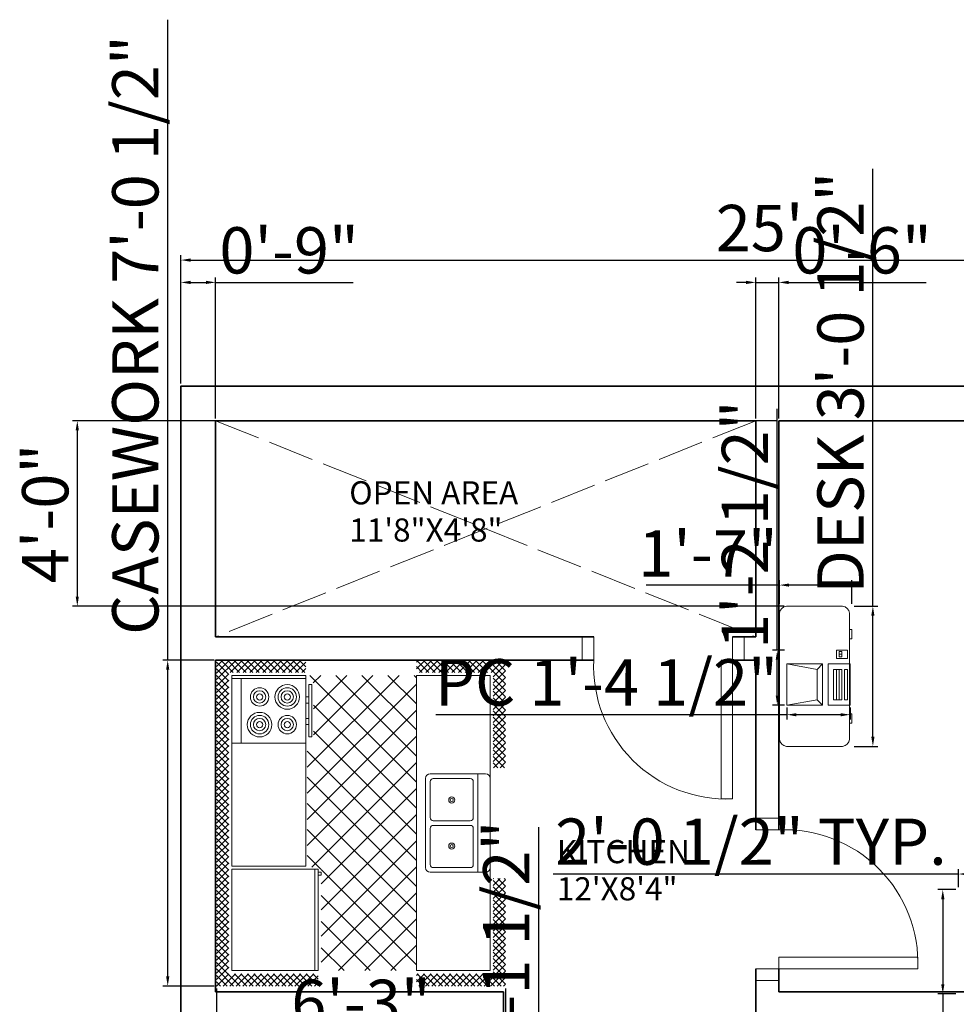
# Model space of a CAD drawing. Units: inches. Extents: x 2446 to 3341, y 462 to 1195.
# Tile 3 of 6: x 2503 to 2746, y 888 to 1143. Entities that reach past the tile are written whole.
import ezdxf

# ---------------------------------------------------------------- set-up
doc = ezdxf.new("R2010")
doc.units = ezdxf.units.IN
doc.linetypes.add('ACAD_ISO02W100', pattern=[15, 12, -3])
for name, color, linetype, lineweight in [('A-ANNO-DIMS', 2, 'Continuous', 18), ('A-AREA-IDEN', 7, 'Continuous', 18), ('A-DOOR', 4, 'Continuous', 18), ('A-EQPM', 9, 'Continuous', 18), ('A-FLOR-FIXT', 9, 'Continuous', 18), ('A-FLOR-OPEN', 8, 'ACAD_ISO02W100', 13), ('A-FURN', 8, 'Continuous', 18), ('A-WALL', 7, 'Continuous', 35), ('C-PROP', 7, 'Continuous', 35)]:
    doc.layers.add(name, color=color, linetype=linetype, lineweight=lineweight)
doc.styles.get("Standard").update_dxf_attribs({"font": 'arial.ttf'})
doc.dimstyles.new('ISO-25', dxfattribs={"dimtxt": 12, "dimasz": 2.5, "dimexe": 1.25, "dimexo": 0.625, "dimtad": 1, "dimdec": 1, "dimlunit": 3, "dimtxsty": 'Standard', "dimcen": 2.5, "dimadec": 0, "dimazin": 0, "dimtfac": 1, "dimtdec": 1, "dimtmove": 0, "dimatfit": 3, "dimfxl": 1, "dimarcsym": 0})

# ---------------------------------------------------------------- blocks, each defined once
blk = doc.blocks.new('Desk - 30 x 60 in.')
for p, q in [((-26.999995, 0), (26.999995, 0)), ((-29.999995, -27), (-29.999995, -3)), ((29.999995, -3), (29.999995, -27)), ((26.999995, -30), (-26.999995, -30)), ((-20.000005, -30), (-20.000005, -31)), ((-20.000005, -31), (-16.000005, -31)), ((-16.000005, -31), (-16.000005, -30)), ((15.999995, -31), (15.999995, -30)), ((19.999995, -31), (15.999995, -31)), ((19.999995, -30), (19.999995, -31))]:
    blk.add_line(p, q)
for centre, start, end in [((-26.499995, -3.5), 98.1301, 171.8699), ((26.499995, -3.5), 8.130102, 81.8699), ((-26.499995, -26.5), 188.1301, 261.8699), ((26.499995, -26.5), 278.1301, 351.8699)]:
    blk.add_arc(centre, 3.535534, start, end)
blk = doc.blocks.new('Computer Terminal')
for p, q in [((-10, 11.5), (5, 11.5)), ((-8, 0.5), (-10, 11.5)), ((-10, -1.5), (-10, 11.5)), ((5, 11.5), (3, 0.5)), ((5, 11.5), (5, -1.5)), ((-10, -1.5), (-8, 0.5)), ((3, 0.5), (-8, 0.5)), ((3, 0.5), (5, -1.5)), ((5, -1.5), (-10, -1.5)), ((-10, -11.5), (-10, -3.5)), ((-10, -3.5), (5, -3.5)), ((5, -3.5), (5, -11.5)), ((-8, -5.5), (-8, -8.5)), ((3, -5.5), (-8, -5.5)), ((3, -6.5), (-8, -6.5)), ((3, -8.5), (3, -5.5)), ((10, -6.5), (7, -6.5)), ((7, -6.5), (7, -10.5)), ((10, -10.5), (10, -6.5)), ((-8, -7.5), (3, -7.5)), ((-8, -8.5), (3, -8.5)), ((-8, -9.5), (-8, -10.5)), ((3, -9.5), (-8, -9.5)), ((-8, -10.5), (3, -10.5)), ((3, -10.5), (3, -9.5)), ((7, -10.5), (10, -10.5)), ((9.5, -7.5), (7.5, -7.5)), ((7.5, -7.5), (7.5, -8.5)), ((7.5, -8.5), (9.5, -8.5)), ((8.5, -7.5), (8.5, -8.5)), ((9.5, -8.5), (9.5, -7.5)), ((5, -11.5), (-10, -11.5))]:
    blk.add_line(p, q)
blk = doc.blocks.new('Kitchen Layout - 7 x 8 ft')
for p, q in [((-5, 81.32), (2.68, 89)), ((-5, 83.44), (0.56, 89)), ((-5, 85.56), (-1.56, 89)), ((-5, 87.68), (-3.68, 89)), ((-1, 84.97), (-5, 88.97)), ((-1, 82.85), (-5, 86.85)), ((1.09, 85), (-2.91, 89)), ((3.21, 85), (-0.79, 89)), ((0.81, 85), (4.81, 89)), ((5.34, 85), (1.34, 89)), ((2.93, 85), (6.93, 89)), ((7.46, 85), (3.46, 89)), ((5.05, 85), (9.05, 89)), ((9.58, 85), (5.58, 89)), ((7.17, 85), (11.17, 89)), ((11.7, 85), (7.7, 89)), ((9.29, 85), (13.29, 89)), ((13.82, 85), (9.82, 89)), ((11.41, 85), (15.41, 89)), ((15.94, 85), (11.94, 89)), ((13.53, 85), (17.53, 89)), ((18.06, 85), (14.06, 89)), ((15.65, 85), (19.65, 89)), ((20.18, 85), (16.18, 89)), ((17.78, 85), (21.78, 89)), ((22.31, 85), (18.31, 89)), ((19.9, 85), (23.9, 89)), ((24.43, 85), (20.43, 89)), ((22.02, 85), (26.02, 89)), ((26.55, 85), (22.55, 89)), ((24.14, 85), (28.14, 89)), ((28.67, 85), (24.67, 89)), ((26.26, 85), (30.26, 89)), ((30.79, 85), (26.79, 89)), ((28.38, 85), (32.38, 89)), ((32.91, 85), (28.91, 89)), ((30.5, 85), (34.5, 89)), ((35.03, 85), (31.03, 89)), ((32.63, 85), (36.63, 89)), ((37.16, 85), (33.16, 89)), ((34.75, 85), (38.75, 89)), ((39.28, 85), (35.28, 89)), ((36.87, 85), (40.87, 89)), ((41.4, 85), (37.4, 89)), ((38.99, 85), (42.99, 89)), ((43.52, 85), (39.52, 89)), ((41.11, 85), (45.11, 89)), ((45.64, 85), (41.64, 89)), ((43.23, 85), (47.23, 89)), ((47.76, 85), (43.76, 89)), ((45.35, 85), (49.35, 89)), ((49.88, 85), (45.88, 89)), ((47.47, 85), (51.47, 89)), ((52, 85), (48, 89)), ((49.6, 85), (53.6, 89)), ((54.13, 85), (50.13, 89)), ((51.72, 85), (55.72, 89)), ((56.25, 85), (52.25, 89)), ((53.84, 85), (57.84, 89)), ((58.37, 85), (54.37, 89)), ((55.96, 85), (59.96, 89)), ((60.49, 85), (56.49, 89)), ((58.08, 85), (62.08, 89)), ((62.61, 85), (58.61, 89)), ((60.2, 85), (64.2, 89)), ((64.73, 85), (60.73, 89)), ((62.32, 85), (66.32, 89)), ((66.85, 85), (62.85, 89)), ((64.45, 85), (68.45, 89)), ((68.97, 85), (64.97, 89)), ((66.57, 85), (70.57, 89)), ((71.1, 85), (67.1, 89)), ((68.69, 85), (72.69, 89)), ((73.22, 85), (69.22, 89)), ((70.81, 85), (74.81, 89)), ((75.34, 85), (71.34, 89)), ((72.93, 85), (76.93, 89)), ((77.46, 85), (73.46, 89)), ((75.05, 85), (79.05, 89)), ((79.58, 85), (75.58, 89)), ((77.17, 85), (81.17, 89)), ((81.7, 85), (77.7, 89)), ((79.29, 85), (83.29, 89)), ((83.82, 85), (79.82, 89)), ((81.42, 85), (85.42, 89)), ((85.95, 85), (81.95, 89)), ((83.54, 85), (87.54, 89)), ((88.07, 85), (84.07, 89)), ((85.66, 85), (89.66, 89)), ((90.19, 85), (86.19, 89)), ((87.78, 85), (91.78, 89)), ((92.31, 85), (88.31, 89)), ((89.9, 85), (93.9, 89)), ((94.43, 85), (90.43, 89)), ((92.02, 85), (96.02, 89)), ((96.55, 85), (92.55, 89)), ((94.14, 85), (98.14, 89)), ((101, 82.67), (94.67, 89)), ((96.27, 85), (100.27, 89)), ((101, 84.79), (96.79, 89)), ((97, 83.61), (101, 87.61)), ((101, 86.92), (98.92, 89)), ((-1, 80.73), (-5, 84.73)), ((34, 84), (96, 84)), ((34, 60), (34, 84)), ((96, 84), (96, 60)), ((97, 81.49), (101, 85.49)), ((101, 80.55), (97, 84.55)), ((97, 79.37), (101, 83.37)), ((-5, 79.19), (-1, 83.19)), ((-1, 78.61), (-5, 82.61)), ((-5, 77.07), (-1, 81.07)), ((-1, 76.49), (-5, 80.49)), ((74, 81), (95, 81)), ((101, 78.43), (97, 82.43)), ((97, 77.25), (101, 81.25)), ((101, 76.31), (97, 80.31)), ((-5, 74.95), (-1, 78.95)), ((-1, 74.36), (-5, 78.36)), ((97, 75.13), (101, 79.13)), ((101, 74.19), (97, 78.19)), ((97, 73.01), (101, 77.01)), ((-5, 72.83), (-1, 76.83)), ((-1, 72.24), (-5, 76.24)), ((-5, 70.71), (-1, 74.71)), ((-1, 70.12), (-5, 74.12)), ((101, 72.07), (97, 76.07)), ((97, 70.89), (101, 74.89)), ((101, 69.95), (97, 73.95)), ((-5, 68.59), (-1, 72.59)), ((-1, 68), (-5, 72)), ((-5, 66.47), (-1, 70.47)), ((97, 68.76), (101, 72.76)), ((101, 67.82), (97, 71.82)), ((97, 66.64), (101, 70.64)), ((-1, 65.88), (-5, 69.88)), ((-5, 64.35), (-1, 68.35)), ((-1, 63.76), (-5, 67.76)), ((101, 65.7), (97, 69.7)), ((97, 64.52), (101, 68.52)), ((101, 63.58), (97, 67.58)), ((-5, 62.22), (-1, 66.22)), ((-1, 61.64), (-5, 65.64)), ((-5, 60.1), (-1, 64.1)), ((97, 62.4), (101, 66.4)), ((101, 61.46), (97, 65.46)), ((97, 60.28), (101, 64.28)), ((-1, 59.52), (-5, 63.52)), ((-5, 57.98), (-1, 61.98)), ((-1, 57.39), (-5, 61.39)), ((100.34, 60), (97, 63.34)), ((98.22, 60), (97, 61.22)), ((98.84, 60), (101, 62.16)), ((-1.73, 56), (-5, 59.27)), ((-4.86, 56), (-1, 59.86)), ((-2.74, 56), (-1, 57.74)), ((10.4, 24), (45.9, 59.5)), ((18.88, 24), (54.38, 59.5)), ((27.37, 24), (62.87, 59.5)), ((33.03, 55.11), (37.41, 59.5)), ((67.71, 24), (33.68, 58.04)), ((96, 60), (34, 60)), ((35.85, 24), (71.35, 59.5)), ((76.2, 24), (40.7, 59.5)), ((84.68, 24), (49.18, 59.5)), ((93.17, 24), (57.67, 59.5)), ((61.31, 24), (96, 58.69)), ((96, 29.65), (66.15, 59.5)), ((80, 60), (80, 59)), ((82, 59), (82, 60)), ((87, 59), (87, 60)), ((89, 60), (89, 59)), ((100.96, 60), (101, 60.04)), ((-3.85, 56), (-5, 57.15)), ((0, 57), (33, 57)), ((0, 30.57), (24.43, 55)), ((0, 39.06), (15.94, 55)), ((0, 47.54), (7.46, 55)), ((1.91, 24), (32.91, 55)), ((33.77, 24), (2.77, 55)), ((42.26, 24), (11.26, 55)), ((50.74, 24), (19.74, 55)), ((59.23, 24), (28.23, 55)), ((31, 55), (31, 56)), ((32, 55), (31, 55)), ((32, 56), (32, 55)), ((44.34, 24), (77.84, 57.5)), ((52.82, 24), (86.32, 57.5)), ((96, 38.14), (76.64, 57.5)), ((96, 46.63), (85.13, 57.5)), ((96, 55.11), (93.57, 57.54)), ((25.29, 24), (0, 49.29)), ((69.79, 24), (96, 50.21)), ((78.28, 24), (96, 41.72)), ((16.8, 24), (0, 40.8)), ((8.32, 24), (0, 32.32)), ((86.76, 24), (96, 33.24)), ((-5, 21.92), (-2.92, 24)), ((-5, 19.8), (-1, 23.8)), ((-1, 19.21), (-5, 23.21)), ((-1, 21.33), (-3.67, 24)), ((-1, 23.45), (-1.55, 24)), ((0, 24), (96, 24)), ((0, 0), (0, 24)), ((95.25, 24), (96, 24.75)), ((96, 24), (96, 0)), ((97, 22.1), (98.9, 24)), ((97, 19.97), (101, 23.97)), ((101, 19.03), (97, 23.03)), ((101, 21.16), (98.16, 24)), ((101, 23.28), (100.28, 24)), ((-5, 17.68), (-1, 21.68)), ((-1, 17.09), (-5, 21.09)), ((-5, 15.55), (-1, 19.55)), ((97, 17.85), (101, 21.85)), ((101, 16.91), (97, 20.91)), ((97, 15.73), (101, 19.73)), ((-1, 14.97), (-5, 18.97)), ((-5, 13.43), (-1, 17.43)), ((-1, 12.85), (-5, 16.85)), ((47.25, 6.5), (47.25, 18.5)), ((48.75, 18.5), (48.75, 6.5)), ((101, 14.79), (97, 18.79)), ((97, 13.61), (101, 17.61)), ((101, 12.67), (97, 16.67)), ((-5, 11.31), (-1, 15.31)), ((-1, 10.73), (-5, 14.73)), ((-5, 9.19), (-1, 13.19)), ((97, 11.49), (101, 15.49)), ((101, 10.55), (97, 14.55)), ((97, 9.37), (101, 13.37)), ((-1, 8.6), (-5, 12.6)), ((-5, 7.07), (-1, 11.07)), ((-1, 6.48), (-5, 10.48)), ((101, 8.43), (97, 12.43)), ((97, 7.25), (101, 11.25)), ((101, 6.31), (97, 10.31)), ((-5, 4.95), (-1, 8.95)), ((-1, 4.36), (-5, 8.36)), ((-5, 2.83), (-1, 6.83)), ((97, 5.12), (101, 9.12)), ((101, 4.18), (97, 8.18)), ((97, 3), (101, 7)), ((-1, 2.24), (-5, 6.24)), ((-5, 0.71), (-1, 4.71)), ((-1, 0.12), (-5, 4.12)), ((64, 4), (32, 4)), ((101, 2.06), (97, 6.06)), ((97, 0.88), (101, 4.88)), ((101, -0.06), (97, 3.94)), ((-5, -1.42), (-1, 2.58)), ((2, -5), (-5, 2)), ((-5, -3.54), (-1, 0.46)), ((96, 0), (0, 0)), ((93.24, -5), (101, 2.76)), ((95.36, -5), (101, 0.64)), ((101, -2.18), (97, 1.82)), ((-0.12, -5), (-5, -0.12)), ((-2.25, -5), (-5, -2.25)), ((-4.34, -5), (-0.34, -1)), ((-2.22, -5), (1.78, -1)), ((-0.1, -5), (3.9, -1)), ((4.12, -5), (0.12, -1)), ((2.02, -5), (6.02, -1)), ((6.24, -5), (2.24, -1)), ((4.14, -5), (8.14, -1)), ((8.36, -5), (4.36, -1)), ((6.27, -5), (10.27, -1)), ((10.48, -5), (6.48, -1)), ((8.39, -5), (12.39, -1)), ((12.6, -5), (8.6, -1)), ((10.51, -5), (14.51, -1)), ((14.73, -5), (10.73, -1)), ((12.63, -5), (16.63, -1)), ((16.85, -5), (12.85, -1)), ((14.75, -5), (18.75, -1)), ((18.97, -5), (14.97, -1)), ((16.87, -5), (20.87, -1)), ((21.09, -5), (17.09, -1)), ((18.99, -5), (22.99, -1)), ((23.21, -5), (19.21, -1)), ((21.11, -5), (25.11, -1)), ((25.33, -5), (21.33, -1)), ((23.24, -5), (27.24, -1)), ((27.45, -5), (23.45, -1)), ((25.36, -5), (29.36, -1)), ((29.57, -5), (25.57, -1)), ((27.48, -5), (30, -2.48)), ((30, -3.3), (27.7, -1)), ((30, -1.18), (29.82, -1)), ((66, -2.54), (67.54, -1)), ((66, -4.66), (69.66, -1)), ((69.88, -5), (66, -1.12)), ((67.78, -5), (71.78, -1)), ((72, -5), (68, -1)), ((69.9, -5), (73.9, -1)), ((74.12, -5), (70.12, -1)), ((72.03, -5), (76.03, -1)), ((76.24, -5), (72.24, -1)), ((74.15, -5), (78.15, -1)), ((78.36, -5), (74.36, -1)), ((76.27, -5), (80.27, -1)), ((80.49, -5), (76.49, -1)), ((78.39, -5), (82.39, -1)), ((82.61, -5), (78.61, -1)), ((80.51, -5), (84.51, -1)), ((84.73, -5), (80.73, -1)), ((82.63, -5), (86.63, -1)), ((86.85, -5), (82.85, -1)), ((84.75, -5), (88.75, -1)), ((88.97, -5), (84.97, -1)), ((86.88, -5), (90.88, -1)), ((91.09, -5), (87.09, -1)), ((89, -5), (93, -1)), ((93.21, -5), (89.21, -1)), ((91.12, -5), (95.12, -1)), ((95.34, -5), (91.34, -1)), ((97.46, -5), (93.46, -1)), ((99.58, -5), (95.58, -1)), ((101, -4.3), (97, -0.3)), ((97.48, -5), (101, -1.48)), ((-4.37, -5), (-5, -4.37)), ((29.6, -5), (30, -4.6)), ((67.76, -5), (66, -3.24)), ((99.6, -5), (101, -3.6))]:
    blk.add_line(p, q)
for points in [[(0, 56), (0, 84), (33, 84), (33, 56)], [(74, 60), (74, 84), (95, 84), (95, 60)], [(76, 58), (76, 59), (93, 59), (93, 58)]]:
    blk.add_lwpolyline(points, close=True)
for points in [[(32, 1.5), (32, 19.5)], [(33.5, 21), (62.5, 21)], [(34.5, 19.5), (46.25, 19.5)], [(49.75, 19.5), (61.5, 19.5)], [(64, 19.5), (64, 1.5)], [(33.5, 6.5), (33.5, 18.5)], [(62.5, 18.5), (62.5, 6.5)], [(46.25, 5.5), (34.5, 5.5)], [(61.5, 5.5), (49.75, 5.5)], [(62.5, 0), (33.5, 0)]]:
    blk.add_lwpolyline(points)
for centre, radius in [((80, 75), 4), ((80, 75), 3), ((80, 75), 2), ((89, 75), 3), ((89, 75), 2), ((80, 75), 1), ((89, 75), 1), ((80, 66), 3), ((80, 66), 2), ((89, 66), 4), ((89, 66), 3), ((89, 66), 2), ((80, 66), 1), ((89, 66), 1), ((40.5, 12.5), 1), ((40.5, 12.5), 0.5), ((55.5, 12.5), 1), ((55.5, 12.5), 0.5)]:
    blk.add_circle(centre, radius)
for centre, radius, start, end in [((33.5, 19.5), 1.5, 90, 180), ((34.5, 18.5), 1, 90, 180), ((46.25, 18.5), 1, 0, 90), ((49.75, 18.5), 1, 90, 180), ((61.5, 18.5), 1, 0, 90), ((62.5, 19.5), 1.5, 0, 90), ((34.5, 6.5), 1, 180, 270), ((46.25, 6.5), 1, 270, 0), ((49.75, 6.5), 1, 180, 270), ((61.5, 6.5), 1, 270, 0), ((33.5, 1.5), 1.5, 180, 270), ((62.5, 1.5), 1.5, 270, 0)]:
    blk.add_arc(centre, radius, start, end)
blk = doc.blocks.new('*D17')
at = {"layer": 'A-ANNO-DIMS', "color": 0, "lineweight": -2, "transparency": 16777216}
for p, q in [((2544.62, 1048.59), (2544.62, 1081.85)), ((2844.62, 1048.59), (2844.62, 1081.85)), ((2547.12, 1080.6), (2842.12, 1080.6))]:
    blk.add_line(p, q, dxfattribs=at)
at = {"layer": 'A-ANNO-DIMS', "color": 0, "transparency": 16777216}
for points in [[(2547.12, 1081.02), (2547.12, 1080.18), (2544.62, 1080.6)], [(2842.12, 1081.02), (2842.12, 1080.18), (2844.62, 1080.6)]]:
    blk.add_solid(points, dxfattribs=at)
at = {"layer": 'Defpoints', "color": 0, "transparency": 16777216}
for p in [(2844.62, 1080.6), (2544.62, 1047.97), (2844.62, 1047.97)]:
    blk.add_point(p, dxfattribs=at)
at = {"layer": 'A-ANNO-DIMS', "color": 0, "transparency": 16777216, "insert": (2694.62, 1087.35), "char_height": 12, "attachment_point": 5}
blk.add_mtext("25'", dxfattribs=at)
blk = doc.blocks.new('DOOR-SWING-36IN')
for p, q in [((6, 42), (0, 42)), ((6, 39), (0, 39)), ((6, 3), (0, 3)), ((6, 0), (0, 0))]:
    blk.add_line(p, q)
blk.add_lwpolyline([(6, 3), (42, 3), (42, 6), (6, 6)], close=True)
blk.add_arc((7.5, 4.5), 34.53, 357.5104, 92.4896)
blk = doc.blocks.new('*D33')
at = {"layer": 'A-ANNO-DIMS', "color": 0, "lineweight": -2, "transparency": 16777216}
for p, q in [((2745.53, 917.47), (2740.86, 917.47)), ((2742.11, 914.97), (2742.11, 892.97)), ((2745.53, 890.47), (2740.86, 890.47)), ((2742.11, 890.47), (2742.11, 737.82))]:
    blk.add_line(p, q, dxfattribs=at)
at = {"layer": 'A-ANNO-DIMS', "color": 0, "transparency": 16777216}
for points in [[(2741.69, 914.97), (2742.53, 914.97), (2742.11, 917.47)], [(2741.69, 892.97), (2742.53, 892.97), (2742.11, 890.47)]]:
    blk.add_solid(points, dxfattribs=at)
at = {"layer": 'Defpoints', "color": 0, "transparency": 16777216}
for p in [(2746.16, 917.47), (2742.11, 890.47), (2746.16, 890.47)]:
    blk.add_point(p, dxfattribs=at)
at = {"layer": 'A-ANNO-DIMS', "color": 0, "transparency": 16777216, "insert": (2735.27, 812.89), "char_height": 12, "attachment_point": 5, "rotation": 90}
blk.add_mtext('ROCKER 2\'-3" TYP.', dxfattribs=at)
blk = doc.blocks.new('*D34')
at = {"layer": 'A-ANNO-DIMS', "color": 0, "lineweight": -2, "transparency": 16777216}
for p, q in [((2746.16, 921.52), (2641.1, 921.52)), ((2746.16, 918.09), (2746.16, 922.77)), ((2768.09, 921.52), (2748.66, 921.52)), ((2770.59, 918.09), (2770.59, 922.77))]:
    blk.add_line(p, q, dxfattribs=at)
at = {"layer": 'A-ANNO-DIMS', "color": 0, "transparency": 16777216}
for points in [[(2748.66, 921.94), (2748.66, 921.1), (2746.16, 921.52)], [(2768.09, 921.94), (2768.09, 921.1), (2770.59, 921.52)]]:
    blk.add_solid(points, dxfattribs=at)
at = {"layer": 'Defpoints', "color": 0, "transparency": 16777216}
for p in [(2746.16, 921.52), (2746.16, 917.47), (2770.59, 917.47)]:
    blk.add_point(p, dxfattribs=at)
at = {"layer": 'A-ANNO-DIMS', "color": 0, "transparency": 16777216, "insert": (2692.38, 928.35), "char_height": 12, "attachment_point": 5}
blk.add_mtext('2\'-0 1/2" TYP.', dxfattribs=at)
blk = doc.blocks.new('*D41')
at = {"layer": 'A-ANNO-DIMS', "color": 0, "lineweight": -2, "transparency": 16777216}
for p, q in [((2723.99, 990.93), (2723.99, 1104.25)), ((2719.16, 990.93), (2725.24, 990.93)), ((2723.99, 957.09), (2723.99, 988.43)), ((2719.16, 954.59), (2725.24, 954.59))]:
    blk.add_line(p, q, dxfattribs=at)
at = {"layer": 'A-ANNO-DIMS', "color": 0, "transparency": 16777216}
for points in [[(2723.57, 988.43), (2724.4, 988.43), (2723.99, 990.93)], [(2723.57, 957.09), (2724.4, 957.09), (2723.99, 954.59)]]:
    blk.add_solid(points, dxfattribs=at)
at = {"layer": 'Defpoints', "color": 0, "transparency": 16777216}
for p in [(2718.54, 990.93), (2723.99, 990.93), (2718.54, 954.59)]:
    blk.add_point(p, dxfattribs=at)
at = {"layer": 'A-ANNO-DIMS', "color": 0, "transparency": 16777216, "insert": (2717.15, 1048.84), "char_height": 12, "attachment_point": 5, "rotation": 90}
blk.add_mtext('DESK 3\'-0 1/2"', dxfattribs=at)
blk = doc.blocks.new('*D42')
at = {"layer": 'A-ANNO-DIMS', "color": 0, "lineweight": -2, "transparency": 16777216}
for p, q in [((2699.76, 991.56), (2699.76, 997.64)), ((2718.54, 991.56), (2718.54, 997.64)), ((2699.76, 996.39), (2665.24, 996.39)), ((2716.04, 996.39), (2702.26, 996.39))]:
    blk.add_line(p, q, dxfattribs=at)
at = {"layer": 'A-ANNO-DIMS', "color": 0, "transparency": 16777216}
for points in [[(2702.26, 996.8), (2702.26, 995.97), (2699.76, 996.39)], [(2716.04, 996.8), (2716.04, 995.97), (2718.54, 996.39)]]:
    blk.add_solid(points, dxfattribs=at)
at = {"layer": 'Defpoints', "color": 0, "transparency": 16777216}
for p in [(2699.76, 996.39), (2699.76, 990.93), (2718.54, 990.93)]:
    blk.add_point(p, dxfattribs=at)
at = {"layer": 'A-ANNO-DIMS', "color": 0, "transparency": 16777216, "insert": (2681.25, 1003.03), "char_height": 12, "attachment_point": 5}
blk.add_mtext('1\'-7"', dxfattribs=at)
blk = doc.blocks.new('*D45')
at = {"layer": 'A-ANNO-DIMS', "color": 0, "lineweight": -2, "transparency": 16777216}
for p, q in [((2701.68, 964.63), (2701.68, 961.55)), ((2718.1, 964.63), (2718.1, 961.55)), ((2701.68, 962.8), (2610.72, 962.8)), ((2715.6, 962.8), (2704.18, 962.8))]:
    blk.add_line(p, q, dxfattribs=at)
at = {"layer": 'A-ANNO-DIMS', "color": 0, "transparency": 16777216}
for points in [[(2704.18, 963.21), (2704.18, 962.38), (2701.68, 962.8)], [(2715.6, 963.21), (2715.6, 962.38), (2718.1, 962.8)]]:
    blk.add_solid(points, dxfattribs=at)
at = {"layer": 'Defpoints', "color": 0, "transparency": 16777216}
for p in [(2701.68, 965.26), (2718.1, 965.26), (2701.68, 962.8)]:
    blk.add_point(p, dxfattribs=at)
at = {"layer": 'A-ANNO-DIMS', "color": 0, "transparency": 16777216, "insert": (2654.95, 969.63), "char_height": 12, "attachment_point": 5}
blk.add_mtext('PC 1\'-4 1/2"', dxfattribs=at)
blk = doc.blocks.new('*D46')
at = {"layer": 'A-ANNO-DIMS', "color": 0, "lineweight": -2, "transparency": 16777216}
for p, q in [((2699.21, 979.54), (2699.21, 1042.02)), ((2701.05, 979.54), (2697.96, 979.54)), ((2699.21, 967.76), (2699.21, 977.04)), ((2701.05, 965.26), (2697.96, 965.26))]:
    blk.add_line(p, q, dxfattribs=at)
at = {"layer": 'A-ANNO-DIMS', "color": 0, "transparency": 16777216}
for points in [[(2698.8, 977.04), (2699.63, 977.04), (2699.21, 979.54)], [(2698.8, 967.76), (2699.63, 967.76), (2699.21, 965.26)]]:
    blk.add_solid(points, dxfattribs=at)
at = {"layer": 'Defpoints', "color": 0, "transparency": 16777216}
for p in [(2699.21, 979.54), (2701.68, 979.54), (2701.68, 965.26)]:
    blk.add_point(p, dxfattribs=at)
at = {"layer": 'A-ANNO-DIMS', "color": 0, "transparency": 16777216, "insert": (2692.38, 1012.03), "char_height": 12, "attachment_point": 5, "rotation": 90}
blk.add_mtext('1\'-2 1/2"', dxfattribs=at)
blk = doc.blocks.new('*D54')
at = {"layer": 'A-ANNO-DIMS', "color": 0, "lineweight": -2, "transparency": 16777216}
for p, q in [((2637.36, 870.08), (2637.36, 933.69)), ((2628.68, 870.08), (2638.61, 870.08)), ((2637.36, 835.1), (2637.36, 867.58)), ((2628.68, 832.6), (2638.61, 832.6))]:
    blk.add_line(p, q, dxfattribs=at)
at = {"layer": 'A-ANNO-DIMS', "color": 0, "transparency": 16777216}
for points in [[(2636.94, 867.58), (2637.77, 867.58), (2637.36, 870.08)], [(2636.94, 835.1), (2637.77, 835.1), (2637.36, 832.6)]]:
    blk.add_solid(points, dxfattribs=at)
at = {"layer": 'Defpoints', "color": 0, "transparency": 16777216}
for p in [(2628.06, 870.08), (2637.36, 870.08), (2628.06, 832.6)]:
    blk.add_point(p, dxfattribs=at)
at = {"layer": 'A-ANNO-DIMS', "color": 0, "transparency": 16777216, "insert": (2630.52, 903.14), "char_height": 12, "attachment_point": 5, "rotation": 90}
blk.add_mtext('3\'-1 1/2"', dxfattribs=at)
blk = doc.blocks.new('*D55')
at = {"layer": 'A-ANNO-DIMS', "color": 0, "lineweight": -2, "transparency": 16777216}
for p, q in [((2541.2, 976.96), (2541.2, 1142.89)), ((2553.25, 976.96), (2539.95, 976.96)), ((2541.2, 895), (2541.2, 974.46)), ((2553.25, 892.5), (2539.95, 892.5))]:
    blk.add_line(p, q, dxfattribs=at)
at = {"layer": 'A-ANNO-DIMS', "color": 0, "transparency": 16777216}
for points in [[(2540.79, 974.46), (2541.62, 974.46), (2541.2, 976.96)], [(2540.79, 895), (2541.62, 895), (2541.2, 892.5)]]:
    blk.add_solid(points, dxfattribs=at)
at = {"layer": 'Defpoints', "color": 0, "transparency": 16777216}
for p in [(2541.2, 976.96), (2553.87, 976.96), (2553.87, 892.5)]:
    blk.add_point(p, dxfattribs=at)
at = {"layer": 'A-ANNO-DIMS', "color": 0, "transparency": 16777216, "insert": (2534.37, 1061.18), "char_height": 12, "attachment_point": 5, "rotation": 90}
blk.add_mtext('CASEWORK 7\'-0 1/2"', dxfattribs=at)
blk = doc.blocks.new('*D56')
at = {"layer": 'A-ANNO-DIMS', "color": 0, "lineweight": -2, "transparency": 16777216}
for p, q in [((2553.87, 891.87), (2553.87, 878.58)), ((2628.78, 891.87), (2628.78, 878.58)), ((2626.28, 879.83), (2556.37, 879.83))]:
    blk.add_line(p, q, dxfattribs=at)
at = {"layer": 'A-ANNO-DIMS', "color": 0, "transparency": 16777216}
for points in [[(2556.37, 880.24), (2556.37, 879.41), (2553.87, 879.83)], [(2626.28, 880.24), (2626.28, 879.41), (2628.78, 879.83)]]:
    blk.add_solid(points, dxfattribs=at)
at = {"layer": 'Defpoints', "color": 0, "transparency": 16777216}
for p in [(2553.87, 892.5), (2628.78, 892.5), (2553.87, 879.83)]:
    blk.add_point(p, dxfattribs=at)
at = {"layer": 'A-ANNO-DIMS', "color": 0, "transparency": 16777216, "insert": (2591.32, 886.58), "char_height": 12, "attachment_point": 5}
blk.add_mtext('6\'-3"', dxfattribs=at)
blk = doc.blocks.new('*D67')
at = {"layer": 'A-ANNO-DIMS', "color": 0, "lineweight": -2, "transparency": 16777216}
for p, q in [((2544.62, 1048.59), (2544.62, 1076.07)), ((2547.12, 1074.82), (2551.12, 1074.82)), ((2553.62, 1039.59), (2553.62, 1076.07)), ((2553.62, 1074.82), (2589.27, 1074.82))]:
    blk.add_line(p, q, dxfattribs=at)
at = {"layer": 'A-ANNO-DIMS', "color": 0, "transparency": 16777216}
for points in [[(2547.12, 1075.24), (2547.12, 1074.4), (2544.62, 1074.82)], [(2551.12, 1075.24), (2551.12, 1074.4), (2553.62, 1074.82)]]:
    blk.add_solid(points, dxfattribs=at)
at = {"layer": 'Defpoints', "color": 0, "transparency": 16777216}
for p in [(2553.62, 1074.82), (2544.62, 1047.97), (2553.62, 1038.97)]:
    blk.add_point(p, dxfattribs=at)
at = {"layer": 'A-ANNO-DIMS', "color": 0, "transparency": 16777216, "insert": (2572.69, 1081.57), "char_height": 12, "attachment_point": 5}
blk.add_mtext('0\'-9"', dxfattribs=at)
blk = doc.blocks.new('*D68')
at = {"layer": 'A-ANNO-DIMS', "color": 0, "lineweight": -2, "transparency": 16777216}
for p, q in [((2691.12, 1074.82), (2688.62, 1074.82)), ((2693.62, 1039.59), (2693.62, 1076.07)), ((2693.62, 1074.82), (2699.62, 1074.82)), ((2699.62, 1039.59), (2699.62, 1076.07)), ((2702.12, 1074.82), (2737.77, 1074.82))]:
    blk.add_line(p, q, dxfattribs=at)
at = {"layer": 'A-ANNO-DIMS', "color": 0, "transparency": 16777216}
for points in [[(2691.12, 1075.24), (2691.12, 1074.4), (2693.62, 1074.82)], [(2702.12, 1075.24), (2702.12, 1074.4), (2699.62, 1074.82)]]:
    blk.add_solid(points, dxfattribs=at)
at = {"layer": 'Defpoints', "color": 0, "transparency": 16777216}
for p in [(2699.62, 1074.82), (2693.62, 1038.97), (2699.62, 1038.97)]:
    blk.add_point(p, dxfattribs=at)
at = {"layer": 'A-ANNO-DIMS', "color": 0, "transparency": 16777216, "insert": (2721.19, 1081.57), "char_height": 12, "attachment_point": 5}
blk.add_mtext('0\'-6"', dxfattribs=at)
blk = doc.blocks.new('*D77')
at = {"layer": 'A-ANNO-DIMS', "color": 0, "lineweight": -2, "transparency": 16777216}
for p, q in [((2698.99, 1038.97), (2516.52, 1038.97)), ((2517.77, 1036.47), (2517.77, 993.43)), ((2700.95, 990.93), (2516.52, 990.93))]:
    blk.add_line(p, q, dxfattribs=at)
at = {"layer": 'A-ANNO-DIMS', "color": 0, "transparency": 16777216}
for points in [[(2517.35, 1036.47), (2518.18, 1036.47), (2517.77, 1038.97)], [(2517.35, 993.43), (2518.18, 993.43), (2517.77, 990.93)]]:
    blk.add_solid(points, dxfattribs=at)
at = {"layer": 'Defpoints', "color": 0, "transparency": 16777216}
for p in [(2699.62, 1038.97), (2517.77, 990.93), (2701.57, 990.93)]:
    blk.add_point(p, dxfattribs=at)
at = {"layer": 'A-ANNO-DIMS', "color": 0, "transparency": 16777216, "insert": (2511.01, 1014.95), "char_height": 12, "attachment_point": 5, "rotation": 90}
blk.add_mtext('4\'-0"', dxfattribs=at)

msp = doc.modelspace()

# ---------------------------------------------------------------- linework, layer by layer
at = {"layer": 'A-FLOR-OPEN'}
for p, q in [((2553.62, 1038.97), (2693.62, 982.97)), ((2693.62, 1038.97), (2553.62, 982.97))]:
    msp.add_line(p, q, dxfattribs=at)
at = {"layer": 'A-WALL'}
for p, q in [((2553.62, 1038.97), (2553.62, 982.97)), ((2693.62, 1038.97), (2553.62, 1038.97)), ((2693.62, 1038.97), (2693.62, 982.97)), ((2835.62, 1038.97), (2699.62, 1038.97)), ((2699.62, 1038.97), (2699.62, 932.97)), ((2651.62, 982.97), (2553.62, 982.97)), ((2693.62, 982.97), (2687.62, 982.97)), ((2553.62, 976.97), (2553.62, 890.97)), ((2651.62, 976.97), (2553.62, 976.97)), ((2693.62, 976.97), (2687.62, 976.97)), ((2693.62, 976.97), (2693.62, 932.97)), ((2693.62, 896.97), (2693.62, 890.97)), ((2699.62, 896.97), (2699.62, 890.97)), ((2628.27, 890.97), (2553.62, 890.97)), ((2628.27, 890.97), (2628.27, 884.97)), ((2693.62, 890.97), (2693.62, 884.97)), ((2835.62, 890.97), (2699.62, 890.97))]:
    msp.add_line(p, q, dxfattribs=at)
at = {"layer": 'C-PROP'}
msp.add_lwpolyline([(2544.62, 567.97), (2844.62, 567.97), (2844.62, 1047.97), (2544.62, 1047.97)], close=True, dxfattribs=at)

# ---------------------------------------------------------------- block references
at = {"layer": 'A-DOOR', "extrusion": (0, 0, -1), "zscale": -1, "rotation": 269.999999999998}
msp.add_blockref('DOOR-SWING-36IN', (-2690.62, 982.97), dxfattribs=at)
at = {"layer": 'A-DOOR'}
msp.add_blockref('DOOR-SWING-36IN', (2693.62, 893.97), dxfattribs=at)
at = {"layer": 'A-EQPM', "xscale": 0.7141072854781568, "yscale": 0.7141072854781568, "zscale": 0.7141072854781568, "rotation": 90}
msp.add_blockref('Computer Terminal', (2709.89, 972.4), dxfattribs=at)
at = {"layer": 'A-FLOR-FIXT', "xscale": 0.7968505236229118, "yscale": 0.7968505236229118, "zscale": 0.7968505236229118, "rotation": 90}
msp.add_blockref('Kitchen Layout - 7 x 8 ft', (2624.79, 896.48), dxfattribs=at)
at = {"layer": 'A-FURN', "xscale": 0.6057898034963493, "yscale": 0.6057898034963493, "zscale": 0.6057898034963493, "rotation": 90}
msp.add_blockref('Desk - 30 x 60 in.', (2699.76, 972.76), dxfattribs=at)

# ---------------------------------------------------------------- texts
at = {"layer": 'A-AREA-IDEN'}
for s, p in [('OPEN AREA', (2588.26, 1017.3)), ('11\'8"X4\'8"', (2588.26, 1007.66)), ('KITCHEN', (2642.05, 924.32)), ('12\'X8\'4"', (2642.05, 914.69))]:
    msp.add_text(s, height=6, dxfattribs=at).set_placement(p)

# ---------------------------------------------------------------- dimensions: what is measured, and where the dimension line sits
at = {"layer": 'A-ANNO-DIMS'}
for base, p1, p2, angle, text, picture, middle in [((2541.2, 976.96), (2553.87, 892.5), (2553.87, 976.96), 90, 'CASEWORK <>', '*D55', (2534.37, 1061.18)), ((2723.99, 990.93), (2718.54, 954.59), (2718.54, 990.93), 90, 'DESK <>', '*D41', (2717.15, 1048.84)), ((2701.68, 962.8), (2718.1, 965.26), (2701.68, 965.26), 180, 'PC <>', '*D45', (2654.95, 969.63)), ((2746.16, 921.52), (2770.59, 917.47), (2746.16, 917.47), 180, '<> TYP.', '*D34', (2692.38, 928.35)), ((2742.11, 890.47), (2746.16, 917.47), (2746.16, 890.47), 270, 'ROCKER <> TYP.', '*D33', (2735.27, 812.89))]:
    dim = msp.add_linear_dim(base=base, p1=p1, p2=p2, angle=angle, text=text, dimstyle='ISO-25', override={"dimdec": 1, "dimlfac": 1, "dimrnd": 0, "dimzin": 1, "dimdsep": 46, "dimlunit": 4, "dimfrac": 2}, dxfattribs=at)
    dim.commit()
    dim.dimension.update_dxf_attribs({"geometry": picture, "text_midpoint": middle})
for base, p1, p2, override, picture, middle in [((2844.62, 1080.6), (2544.62, 1047.97), (2844.62, 1047.97), {"dimclrd": 0, "dimclre": 0, "dimclrt": 0}, '*D17', (2694.62, 1087.35)), ((2553.62, 1074.82), (2544.62, 1047.97), (2553.62, 1038.97), {"dimdec": 1, "dimlfac": 1, "dimrnd": 0, "dimzin": 1, "dimdsep": 46, "dimlunit": 4, "dimfrac": 2}, '*D67', (2572.69, 1081.57)), ((2699.62, 1074.82), (2693.62, 1038.97), (2699.62, 1038.97), {"dimdec": 1, "dimlfac": 1, "dimrnd": 0, "dimzin": 1, "dimdsep": 46, "dimlunit": 4, "dimfrac": 2}, '*D68', (2721.19, 1081.57))]:
    dim = msp.add_linear_dim(base=base, p1=p1, p2=p2, dimstyle='ISO-25', override=override, dxfattribs=at)
    dim.commit()
    dim.dimension.update_dxf_attribs({"geometry": picture, "text_midpoint": middle})
for base, p1, p2, angle, picture, middle in [((2699.21, 979.54), (2701.68, 965.26), (2701.68, 979.54), 90, '*D46', (2692.38, 1012.03)), ((2517.77, 990.93), (2699.62, 1038.97), (2701.57, 990.93), 90, '*D77', (2511.01, 1014.95)), ((2699.76, 996.39), (2718.54, 990.93), (2699.76, 990.93), 180, '*D42', (2681.25, 1003.03)), ((2637.36, 870.08), (2628.06, 832.6), (2628.06, 870.08), 90, '*D54', (2630.52, 903.14)), ((2553.87, 879.83), (2628.78, 892.5), (2553.87, 892.5), 180, '*D56', (2591.32, 886.58))]:
    dim = msp.add_linear_dim(base=base, p1=p1, p2=p2, angle=angle, dimstyle='ISO-25', override={"dimdec": 1, "dimlfac": 1, "dimrnd": 0, "dimzin": 1, "dimdsep": 46, "dimlunit": 4, "dimfrac": 2}, dxfattribs=at)
    dim.commit()
    dim.dimension.update_dxf_attribs({"geometry": picture, "text_midpoint": middle})

doc.saveas('drawing.dxf')
